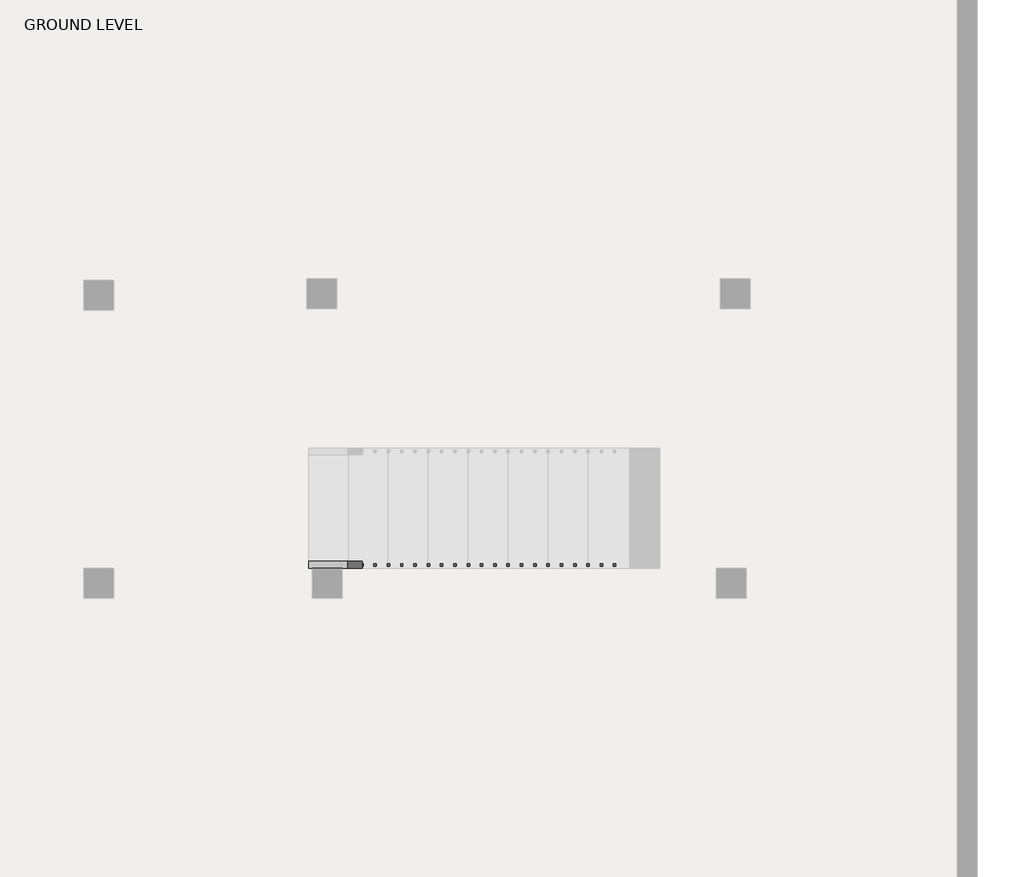
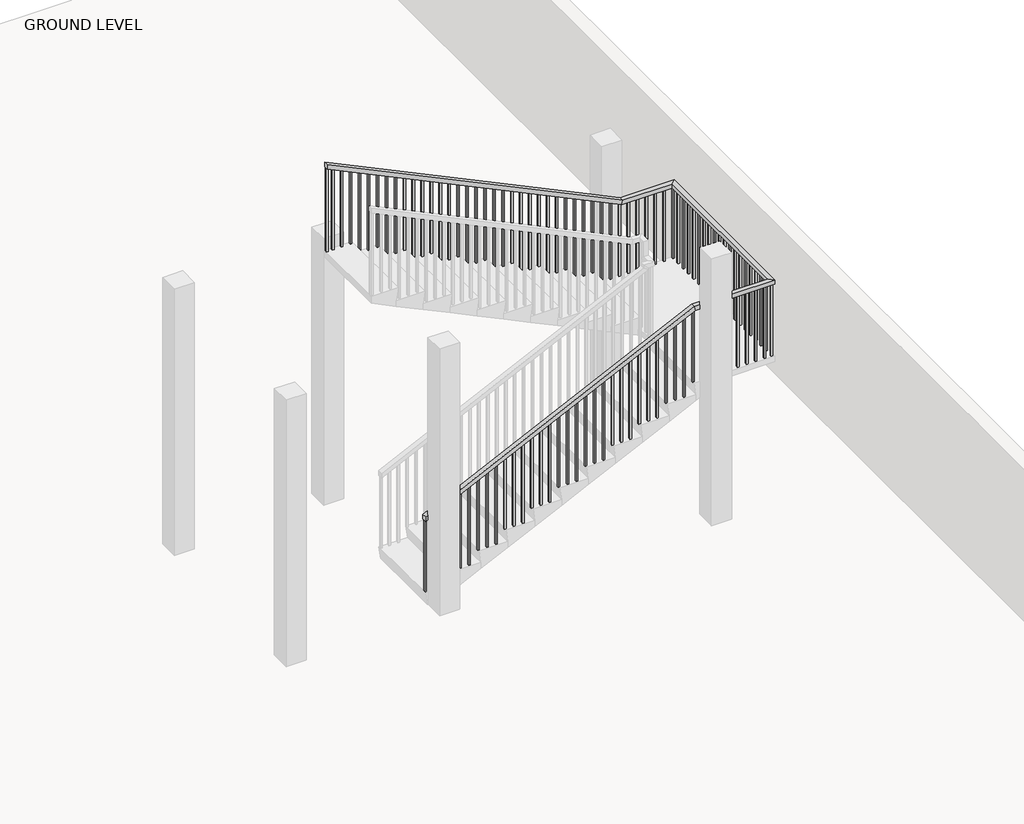
# One storey, part 2 of 3: 1 railing.
"""IFC4 building model written with IfcOpenShell, lengths in millimetres."""

from ifc_helpers import new_model, si_unit, frame, origin, place, context, project, spatial, polyline, outline, extrude, faceted_brep, element, save

model = new_model("IFC4")

# Units and contexts
model_context = context("Model", 3, world=origin())
ifc_project = project(units=[si_unit("LENGTHUNIT", "METRE", prefix="MILLI")], contexts=[model_context])

# Site, building, storey
site = spatial("IfcSite", under=ifc_project)
building = spatial("IfcBuilding", under=site)
storey = spatial("IfcBuildingStorey", under=building, Name="GROUND LEVEL", Elevation=0.0)

# Railing
placement = place(None, origin())
element("IfcRailing", 1, ObjectType="Handrail - Rectangular", at=placement, inside=storey, context=model_context, shape_type="SolidModel", body=[
    faceted_brep([(13.3134019, -453.4212413, 1059.8727273), (13.3134019, -453.4212413, 1003.5834559), (13.3134019, -504.2212413, 1003.5834559), (13.3134019, -504.2212413, 1059.8727273), (3061.3134019, -453.4212413, 2514.6), (3072.8147322, -453.4212413, 2463.8), (3072.8147322, -504.2212413, 2463.8), (3061.3134019, -504.2212413, 2514.6), (3924.9134019, -453.4212413, 2514.6), (3924.9134019, -453.4212413, 2463.8), (3975.7134019, -504.2212413, 2463.8), (3975.7134019, -504.2212413, 2514.6), (3924.9134019, 1426.1787587, 2514.6), (3924.9134019, 1426.1787587, 2463.8), (3975.7134019, 1476.9787587, 2463.8), (3975.7134019, 1476.9787587, 2514.6), (3366.1134019, 1426.1787587, 2514.6), (3354.6120715, 1426.1787587, 2463.8), (3354.6120715, 1476.9787587, 2463.8), (3366.1134019, 1476.9787587, 2514.6), (13.3134019, 1426.1787587, 4114.8), (13.3134019, 1476.9787587, 4114.8), (13.3134019, 1476.9787587, 4058.5107287), (13.3134019, 1426.1787587, 4058.5107287)], [[[0, 1, 2, 3]], [[1, 0, 4, 5]], [[2, 1, 5, 6]], [[3, 2, 6, 7]], [[0, 3, 7, 4]], [[5, 4, 8, 9]], [[6, 5, 9, 10]], [[7, 6, 10, 11]], [[4, 7, 11, 8]], [[9, 8, 12, 13]], [[10, 9, 13, 14]], [[11, 10, 14, 15]], [[8, 11, 15, 12]], [[13, 12, 16, 17]], [[14, 13, 17, 18]], [[15, 14, 18, 19]], [[12, 15, 19, 16]], [[20, 21, 22, 23]], [[17, 16, 20, 23]], [[18, 17, 23, 22]], [[19, 18, 22, 21]], [[16, 19, 21, 20]]]),
    extrude(outline(polyline([(4017.5965241, 99.0384019), (4026.6885696, 79.9884019), (3054.9272727, 79.9884019), (3054.9272727, 99.0384019), (4017.5965241, 99.0384019)])), frame((0.0, 1442.0537587, 0.0), z_axis=(0.0, 1.0, 0.0), x_axis=(0.0, 0.0, 1.0)), (0.0, 0.0, 1.0), 19.05),
    extrude(outline(polyline([(3969.105615, 200.6384019), (3978.1976605, 181.5884019), (3054.9272727, 181.5884019), (3054.9272727, 200.6384019), (3969.105615, 200.6384019)])), frame((0.0, 1442.0537587, 0.0), z_axis=(0.0, 1.0, 0.0), x_axis=(0.0, 0.0, 1.0)), (0.0, 0.0, 1.0), 19.05),
    extrude(outline(polyline([(3920.6147059, 302.2384019), (3929.7067514, 283.1884019), (3054.9272727, 283.1884019), (3054.9272727, 302.2384019), (3920.6147059, 302.2384019)])), frame((0.0, 1442.0537587, 0.0), z_axis=(0.0, 1.0, 0.0), x_axis=(0.0, 0.0, 1.0)), (0.0, 0.0, 1.0), 19.05),
    extrude(outline(polyline([(3872.1237969, 403.8384019), (3881.2158423, 384.7884019), (2909.4545455, 384.7884019), (2909.4545455, 403.8384019), (3872.1237969, 403.8384019)])), frame((0.0, 1442.0537587, 0.0), z_axis=(0.0, 1.0, 0.0), x_axis=(0.0, 0.0, 1.0)), (0.0, 0.0, 1.0), 19.05),
    extrude(outline(polyline([(3823.6328878, 505.4384019), (3832.7249332, 486.3884019), (2909.4545455, 486.3884019), (2909.4545455, 505.4384019), (3823.6328878, 505.4384019)])), frame((0.0, 1442.0537587, 0.0), z_axis=(0.0, 1.0, 0.0), x_axis=(0.0, 0.0, 1.0)), (0.0, 0.0, 1.0), 19.05),
    extrude(outline(polyline([(3775.1419787, 607.0384019), (3784.2340241, 587.9884019), (2909.4545455, 587.9884019), (2909.4545455, 607.0384019), (3775.1419787, 607.0384019)])), frame((0.0, 1442.0537587, 0.0), z_axis=(0.0, 1.0, 0.0), x_axis=(0.0, 0.0, 1.0)), (0.0, 0.0, 1.0), 19.05),
    extrude(outline(polyline([(3726.6510696, 708.6384019), (3735.743115, 689.5884019), (2763.9818182, 689.5884019), (2763.9818182, 708.6384019), (3726.6510696, 708.6384019)])), frame((0.0, 1442.0537587, 0.0), z_axis=(0.0, 1.0, 0.0), x_axis=(0.0, 0.0, 1.0)), (0.0, 0.0, 1.0), 19.05),
    extrude(outline(polyline([(3678.1601605, 810.2384019), (3687.2522059, 791.1884019), (2763.9818182, 791.1884019), (2763.9818182, 810.2384019), (3678.1601605, 810.2384019)])), frame((0.0, 1442.0537587, 0.0), z_axis=(0.0, 1.0, 0.0), x_axis=(0.0, 0.0, 1.0)), (0.0, 0.0, 1.0), 19.05),
    extrude(outline(polyline([(3629.6692514, 911.8384019), (3638.7612969, 892.7884019), (2763.9818182, 892.7884019), (2763.9818182, 911.8384019), (3629.6692514, 911.8384019)])), frame((0.0, 1442.0537587, 0.0), z_axis=(0.0, 1.0, 0.0), x_axis=(0.0, 0.0, 1.0)), (0.0, 0.0, 1.0), 19.05),
    extrude(outline(polyline([(3581.1783423, 1013.4384019), (3590.2703878, 994.3884019), (2618.5090909, 994.3884019), (2618.5090909, 1013.4384019), (3581.1783423, 1013.4384019)])), frame((0.0, 1442.0537587, 0.0), z_axis=(0.0, 1.0, 0.0), x_axis=(0.0, 0.0, 1.0)), (0.0, 0.0, 1.0), 19.05),
    extrude(outline(polyline([(3532.6874332, 1115.0384019), (3541.7794787, 1095.9884019), (2618.5090909, 1095.9884019), (2618.5090909, 1115.0384019), (3532.6874332, 1115.0384019)])), frame((0.0, 1442.0537587, 0.0), z_axis=(0.0, 1.0, 0.0), x_axis=(0.0, 0.0, 1.0)), (0.0, 0.0, 1.0), 19.05),
    extrude(outline(polyline([(3484.1965241, 1216.6384019), (3493.2885696, 1197.5884019), (2618.5090909, 1197.5884019), (2618.5090909, 1216.6384019), (3484.1965241, 1216.6384019)])), frame((0.0, 1442.0537587, 0.0), z_axis=(0.0, 1.0, 0.0), x_axis=(0.0, 0.0, 1.0)), (0.0, 0.0, 1.0), 19.05),
    extrude(outline(polyline([(3435.705615, 1318.2384019), (3444.7976605, 1299.1884019), (2473.0363636, 1299.1884019), (2473.0363636, 1318.2384019), (3435.705615, 1318.2384019)])), frame((0.0, 1442.0537587, 0.0), z_axis=(0.0, 1.0, 0.0), x_axis=(0.0, 0.0, 1.0)), (0.0, 0.0, 1.0), 19.05),
    extrude(outline(polyline([(3387.2147059, 1419.8384019), (3396.3067514, 1400.7884019), (2473.0363636, 1400.7884019), (2473.0363636, 1419.8384019), (3387.2147059, 1419.8384019)])), frame((0.0, 1442.0537587, 0.0), z_axis=(0.0, 1.0, 0.0), x_axis=(0.0, 0.0, 1.0)), (0.0, 0.0, 1.0), 19.05),
    extrude(outline(polyline([(3338.7237969, 1521.4384019), (3347.8158423, 1502.3884019), (2473.0363636, 1502.3884019), (2473.0363636, 1521.4384019), (3338.7237969, 1521.4384019)])), frame((0.0, 1442.0537587, 0.0), z_axis=(0.0, 1.0, 0.0), x_axis=(0.0, 0.0, 1.0)), (0.0, 0.0, 1.0), 19.05),
    extrude(outline(polyline([(3290.2328878, 1623.0384019), (3299.3249332, 1603.9884019), (2327.5636364, 1603.9884019), (2327.5636364, 1623.0384019), (3290.2328878, 1623.0384019)])), frame((0.0, 1442.0537587, 0.0), z_axis=(0.0, 1.0, 0.0), x_axis=(0.0, 0.0, 1.0)), (0.0, 0.0, 1.0), 19.05),
    extrude(outline(polyline([(3241.7419787, 1724.6384019), (3250.8340241, 1705.5884019), (2327.5636364, 1705.5884019), (2327.5636364, 1724.6384019), (3241.7419787, 1724.6384019)])), frame((0.0, 1442.0537587, 0.0), z_axis=(0.0, 1.0, 0.0), x_axis=(0.0, 0.0, 1.0)), (0.0, 0.0, 1.0), 19.05),
    extrude(outline(polyline([(3193.2510696, 1826.2384019), (3202.343115, 1807.1884019), (2327.5636364, 1807.1884019), (2327.5636364, 1826.2384019), (3193.2510696, 1826.2384019)])), frame((0.0, 1442.0537587, 0.0), z_axis=(0.0, 1.0, 0.0), x_axis=(0.0, 0.0, 1.0)), (0.0, 0.0, 1.0), 19.05),
    extrude(outline(polyline([(3144.7601605, 1927.8384019), (3153.8522059, 1908.7884019), (2182.0909091, 1908.7884019), (2182.0909091, 1927.8384019), (3144.7601605, 1927.8384019)])), frame((0.0, 1442.0537587, 0.0), z_axis=(0.0, 1.0, 0.0), x_axis=(0.0, 0.0, 1.0)), (0.0, 0.0, 1.0), 19.05),
    extrude(outline(polyline([(3096.2692514, 2029.4384019), (3105.3612969, 2010.3884019), (2182.0909091, 2010.3884019), (2182.0909091, 2029.4384019), (3096.2692514, 2029.4384019)])), frame((0.0, 1442.0537587, 0.0), z_axis=(0.0, 1.0, 0.0), x_axis=(0.0, 0.0, 1.0)), (0.0, 0.0, 1.0), 19.05),
    extrude(outline(polyline([(3047.7783423, 2131.0384019), (3056.8703878, 2111.9884019), (2182.0909091, 2111.9884019), (2182.0909091, 2131.0384019), (3047.7783423, 2131.0384019)])), frame((0.0, 1442.0537587, 0.0), z_axis=(0.0, 1.0, 0.0), x_axis=(0.0, 0.0, 1.0)), (0.0, 0.0, 1.0), 19.05),
    extrude(outline(polyline([(2999.2874332, 2232.6384019), (3008.3794787, 2213.5884019), (2036.6181818, 2213.5884019), (2036.6181818, 2232.6384019), (2999.2874332, 2232.6384019)])), frame((0.0, 1442.0537587, 0.0), z_axis=(0.0, 1.0, 0.0), x_axis=(0.0, 0.0, 1.0)), (0.0, 0.0, 1.0), 19.05),
    extrude(outline(polyline([(2950.7965241, 2334.2384019), (2959.8885696, 2315.1884019), (2036.6181818, 2315.1884019), (2036.6181818, 2334.2384019), (2950.7965241, 2334.2384019)])), frame((0.0, 1442.0537587, 0.0), z_axis=(0.0, 1.0, 0.0), x_axis=(0.0, 0.0, 1.0)), (0.0, 0.0, 1.0), 19.05),
    extrude(outline(polyline([(2902.305615, 2435.8384019), (2911.3976605, 2416.7884019), (2036.6181818, 2416.7884019), (2036.6181818, 2435.8384019), (2902.305615, 2435.8384019)])), frame((0.0, 1442.0537587, 0.0), z_axis=(0.0, 1.0, 0.0), x_axis=(0.0, 0.0, 1.0)), (0.0, 0.0, 1.0), 19.05),
    extrude(outline(polyline([(2853.8147059, 2537.4384019), (2862.9067514, 2518.3884019), (1891.1454545, 2518.3884019), (1891.1454545, 2537.4384019), (2853.8147059, 2537.4384019)])), frame((0.0, 1442.0537587, 0.0), z_axis=(0.0, 1.0, 0.0), x_axis=(0.0, 0.0, 1.0)), (0.0, 0.0, 1.0), 19.05),
    extrude(outline(polyline([(2805.3237969, 2639.0384019), (2814.4158423, 2619.9884019), (1891.1454545, 2619.9884019), (1891.1454545, 2639.0384019), (2805.3237969, 2639.0384019)])), frame((0.0, 1442.0537587, 0.0), z_axis=(0.0, 1.0, 0.0), x_axis=(0.0, 0.0, 1.0)), (0.0, 0.0, 1.0), 19.05),
    extrude(outline(polyline([(2756.8328878, 2740.6384019), (2765.9249332, 2721.5884019), (1891.1454545, 2721.5884019), (1891.1454545, 2740.6384019), (2756.8328878, 2740.6384019)])), frame((0.0, 1442.0537587, 0.0), z_axis=(0.0, 1.0, 0.0), x_axis=(0.0, 0.0, 1.0)), (0.0, 0.0, 1.0), 19.05),
    extrude(outline(polyline([(2708.3419787, 2842.2384019), (2717.4340241, 2823.1884019), (1745.6727273, 2823.1884019), (1745.6727273, 2842.2384019), (2708.3419787, 2842.2384019)])), frame((0.0, 1442.0537587, 0.0), z_axis=(0.0, 1.0, 0.0), x_axis=(0.0, 0.0, 1.0)), (0.0, 0.0, 1.0), 19.05),
    extrude(outline(polyline([(2659.8510696, 2943.8384019), (2668.943115, 2924.7884019), (1745.6727273, 2924.7884019), (1745.6727273, 2943.8384019), (2659.8510696, 2943.8384019)])), frame((0.0, 1442.0537587, 0.0), z_axis=(0.0, 1.0, 0.0), x_axis=(0.0, 0.0, 1.0)), (0.0, 0.0, 1.0), 19.05),
    extrude(outline(polyline([(2611.3601605, 3045.4384019), (2620.4522059, 3026.3884019), (1745.6727273, 3026.3884019), (1745.6727273, 3045.4384019), (2611.3601605, 3045.4384019)])), frame((0.0, 1442.0537587, 0.0), z_axis=(0.0, 1.0, 0.0), x_axis=(0.0, 0.0, 1.0)), (0.0, 0.0, 1.0), 19.05),
    extrude(outline(polyline([(2562.8692514, 3147.0384019), (2571.9612969, 3127.9884019), (1600.2, 3127.9884019), (1600.2, 3147.0384019), (2562.8692514, 3147.0384019)])), frame((0.0, 1442.0537587, 0.0), z_axis=(0.0, 1.0, 0.0), x_axis=(0.0, 0.0, 1.0)), (0.0, 0.0, 1.0), 19.05),
    extrude(outline(polyline([(2514.3783423, 3248.6384019), (2523.4703878, 3229.5884019), (1600.2, 3229.5884019), (1600.2, 3248.6384019), (2514.3783423, 3248.6384019)])), frame((0.0, 1442.0537587, 0.0), z_axis=(0.0, 1.0, 0.0), x_axis=(0.0, 0.0, 1.0)), (0.0, 0.0, 1.0), 19.05),
    extrude(outline(polyline([(2465.8874332, 3350.2384019), (2474.9794787, 3331.1884019), (1600.2, 3331.1884019), (1600.2, 3350.2384019), (2465.8874332, 3350.2384019)])), frame((0.0, 1442.0537587, 0.0), z_axis=(0.0, 1.0, 0.0), x_axis=(0.0, 0.0, 1.0)), (0.0, 0.0, 1.0), 19.05),
    extrude(outline(polyline([(3451.8384019, 1461.1037587), (3451.8384019, 1442.0537587), (3432.7884019, 1442.0537587), (3432.7884019, 1461.1037587), (3451.8384019, 1461.1037587)])), frame((0.0, 0.0, 1600.2), z_axis=(0.0, 0.0, 1.0), x_axis=(1.0, 0.0, 0.0)), (0.0, 0.0, 1.0), 863.6),
    extrude(outline(polyline([(3553.4384019, 1461.1037587), (3553.4384019, 1442.0537587), (3534.3884019, 1442.0537587), (3534.3884019, 1461.1037587), (3553.4384019, 1461.1037587)])), frame((0.0, 0.0, 1600.2), z_axis=(0.0, 0.0, 1.0), x_axis=(1.0, 0.0, 0.0)), (0.0, 0.0, 1.0), 863.6),
    extrude(outline(polyline([(3655.0384019, 1461.1037587), (3655.0384019, 1442.0537587), (3635.9884019, 1442.0537587), (3635.9884019, 1461.1037587), (3655.0384019, 1461.1037587)])), frame((0.0, 0.0, 1600.2), z_axis=(0.0, 0.0, 1.0), x_axis=(1.0, 0.0, 0.0)), (0.0, 0.0, 1.0), 863.6),
    extrude(outline(polyline([(3756.6384019, 1461.1037587), (3756.6384019, 1442.0537587), (3737.5884019, 1442.0537587), (3737.5884019, 1461.1037587), (3756.6384019, 1461.1037587)])), frame((0.0, 0.0, 1600.2), z_axis=(0.0, 0.0, 1.0), x_axis=(1.0, 0.0, 0.0)), (0.0, 0.0, 1.0), 863.6),
    extrude(outline(polyline([(3858.2384019, 1461.1037587), (3858.2384019, 1442.0537587), (3839.1884019, 1442.0537587), (3839.1884019, 1461.1037587), (3858.2384019, 1461.1037587)])), frame((0.0, 0.0, 1600.2), z_axis=(0.0, 0.0, 1.0), x_axis=(1.0, 0.0, 0.0)), (0.0, 0.0, 1.0), 863.6),
    extrude(outline(polyline([(3959.8384019, 1340.4537587), (3940.7884019, 1340.4537587), (3940.7884019, 1359.5037587), (3959.8384019, 1359.5037587), (3959.8384019, 1340.4537587)])), frame((0.0, 0.0, 1600.2), z_axis=(0.0, 0.0, 1.0), x_axis=(1.0, 0.0, 0.0)), (0.0, 0.0, 1.0), 863.6),
    extrude(outline(polyline([(3959.8384019, 1238.8537587), (3940.7884019, 1238.8537587), (3940.7884019, 1257.9037587), (3959.8384019, 1257.9037587), (3959.8384019, 1238.8537587)])), frame((0.0, 0.0, 1600.2), z_axis=(0.0, 0.0, 1.0), x_axis=(1.0, 0.0, 0.0)), (0.0, 0.0, 1.0), 863.6),
    extrude(outline(polyline([(3959.8384019, 1137.2537587), (3940.7884019, 1137.2537587), (3940.7884019, 1156.3037587), (3959.8384019, 1156.3037587), (3959.8384019, 1137.2537587)])), frame((0.0, 0.0, 1600.2), z_axis=(0.0, 0.0, 1.0), x_axis=(1.0, 0.0, 0.0)), (0.0, 0.0, 1.0), 863.6),
    extrude(outline(polyline([(3959.8384019, 1035.6537587), (3940.7884019, 1035.6537587), (3940.7884019, 1054.7037587), (3959.8384019, 1054.7037587), (3959.8384019, 1035.6537587)])), frame((0.0, 0.0, 1600.2), z_axis=(0.0, 0.0, 1.0), x_axis=(1.0, 0.0, 0.0)), (0.0, 0.0, 1.0), 863.6),
    extrude(outline(polyline([(3959.8384019, 934.0537587), (3940.7884019, 934.0537587), (3940.7884019, 953.1037587), (3959.8384019, 953.1037587), (3959.8384019, 934.0537587)])), frame((0.0, 0.0, 1600.2), z_axis=(0.0, 0.0, 1.0), x_axis=(1.0, 0.0, 0.0)), (0.0, 0.0, 1.0), 863.6),
    extrude(outline(polyline([(3959.8384019, 832.4537587), (3940.7884019, 832.4537587), (3940.7884019, 851.5037587), (3959.8384019, 851.5037587), (3959.8384019, 832.4537587)])), frame((0.0, 0.0, 1600.2), z_axis=(0.0, 0.0, 1.0), x_axis=(1.0, 0.0, 0.0)), (0.0, 0.0, 1.0), 863.6),
    extrude(outline(polyline([(3959.8384019, 730.8537587), (3940.7884019, 730.8537587), (3940.7884019, 749.9037587), (3959.8384019, 749.9037587), (3959.8384019, 730.8537587)])), frame((0.0, 0.0, 1600.2), z_axis=(0.0, 0.0, 1.0), x_axis=(1.0, 0.0, 0.0)), (0.0, 0.0, 1.0), 863.6),
    extrude(outline(polyline([(3959.8384019, 629.2537587), (3940.7884019, 629.2537587), (3940.7884019, 648.3037587), (3959.8384019, 648.3037587), (3959.8384019, 629.2537587)])), frame((0.0, 0.0, 1600.2), z_axis=(0.0, 0.0, 1.0), x_axis=(1.0, 0.0, 0.0)), (0.0, 0.0, 1.0), 863.6),
    extrude(outline(polyline([(3959.8384019, 527.6537587), (3940.7884019, 527.6537587), (3940.7884019, 546.7037587), (3959.8384019, 546.7037587), (3959.8384019, 527.6537587)])), frame((0.0, 0.0, 1600.2), z_axis=(0.0, 0.0, 1.0), x_axis=(1.0, 0.0, 0.0)), (0.0, 0.0, 1.0), 863.6),
    extrude(outline(polyline([(3959.8384019, 426.0537587), (3940.7884019, 426.0537587), (3940.7884019, 445.1037587), (3959.8384019, 445.1037587), (3959.8384019, 426.0537587)])), frame((0.0, 0.0, 1600.2), z_axis=(0.0, 0.0, 1.0), x_axis=(1.0, 0.0, 0.0)), (0.0, 0.0, 1.0), 863.6),
    extrude(outline(polyline([(3959.8384019, 324.4537587), (3940.7884019, 324.4537587), (3940.7884019, 343.5037587), (3959.8384019, 343.5037587), (3959.8384019, 324.4537587)])), frame((0.0, 0.0, 1600.2), z_axis=(0.0, 0.0, 1.0), x_axis=(1.0, 0.0, 0.0)), (0.0, 0.0, 1.0), 863.6),
    extrude(outline(polyline([(3959.8384019, 222.8537587), (3940.7884019, 222.8537587), (3940.7884019, 241.9037587), (3959.8384019, 241.9037587), (3959.8384019, 222.8537587)])), frame((0.0, 0.0, 1600.2), z_axis=(0.0, 0.0, 1.0), x_axis=(1.0, 0.0, 0.0)), (0.0, 0.0, 1.0), 863.6),
    extrude(outline(polyline([(3959.8384019, 121.2537587), (3940.7884019, 121.2537587), (3940.7884019, 140.3037587), (3959.8384019, 140.3037587), (3959.8384019, 121.2537587)])), frame((0.0, 0.0, 1600.2), z_axis=(0.0, 0.0, 1.0), x_axis=(1.0, 0.0, 0.0)), (0.0, 0.0, 1.0), 863.6),
    extrude(outline(polyline([(3959.8384019, 19.6537587), (3940.7884019, 19.6537587), (3940.7884019, 38.7037587), (3959.8384019, 38.7037587), (3959.8384019, 19.6537587)])), frame((0.0, 0.0, 1600.2), z_axis=(0.0, 0.0, 1.0), x_axis=(1.0, 0.0, 0.0)), (0.0, 0.0, 1.0), 863.6),
    extrude(outline(polyline([(3959.8384019, -81.9462413), (3940.7884019, -81.9462413), (3940.7884019, -62.8962413), (3959.8384019, -62.8962413), (3959.8384019, -81.9462413)])), frame((0.0, 0.0, 1600.2), z_axis=(0.0, 0.0, 1.0), x_axis=(1.0, 0.0, 0.0)), (0.0, 0.0, 1.0), 863.6),
    extrude(outline(polyline([(3959.8384019, -183.5462413), (3940.7884019, -183.5462413), (3940.7884019, -164.4962413), (3959.8384019, -164.4962413), (3959.8384019, -183.5462413)])), frame((0.0, 0.0, 1600.2), z_axis=(0.0, 0.0, 1.0), x_axis=(1.0, 0.0, 0.0)), (0.0, 0.0, 1.0), 863.6),
    extrude(outline(polyline([(3959.8384019, -285.1462413), (3940.7884019, -285.1462413), (3940.7884019, -266.0962413), (3959.8384019, -266.0962413), (3959.8384019, -285.1462413)])), frame((0.0, 0.0, 1600.2), z_axis=(0.0, 0.0, 1.0), x_axis=(1.0, 0.0, 0.0)), (0.0, 0.0, 1.0), 863.6),
    extrude(outline(polyline([(3959.8384019, -386.7462413), (3940.7884019, -386.7462413), (3940.7884019, -367.6962413), (3959.8384019, -367.6962413), (3959.8384019, -386.7462413)])), frame((0.0, 0.0, 1600.2), z_axis=(0.0, 0.0, 1.0), x_axis=(1.0, 0.0, 0.0)), (0.0, 0.0, 1.0), 863.6),
    extrude(outline(polyline([(3864.5884019, -488.3462413), (3864.5884019, -469.2962413), (3883.6384019, -469.2962413), (3883.6384019, -488.3462413), (3864.5884019, -488.3462413)])), frame((0.0, 0.0, 1600.2), z_axis=(0.0, 0.0, 1.0), x_axis=(1.0, 0.0, 0.0)), (0.0, 0.0, 1.0), 863.6),
    extrude(outline(polyline([(3762.9884019, -488.3462413), (3762.9884019, -469.2962413), (3782.0384019, -469.2962413), (3782.0384019, -488.3462413), (3762.9884019, -488.3462413)])), frame((0.0, 0.0, 1600.2), z_axis=(0.0, 0.0, 1.0), x_axis=(1.0, 0.0, 0.0)), (0.0, 0.0, 1.0), 863.6),
    extrude(outline(polyline([(3661.3884019, -488.3462413), (3661.3884019, -469.2962413), (3680.4384019, -469.2962413), (3680.4384019, -488.3462413), (3661.3884019, -488.3462413)])), frame((0.0, 0.0, 1600.2), z_axis=(0.0, 0.0, 1.0), x_axis=(1.0, 0.0, 0.0)), (0.0, 0.0, 1.0), 863.6),
    extrude(outline(polyline([(3559.7884019, -488.3462413), (3559.7884019, -469.2962413), (3578.8384019, -469.2962413), (3578.8384019, -488.3462413), (3559.7884019, -488.3462413)])), frame((0.0, 0.0, 1600.2), z_axis=(0.0, 0.0, 1.0), x_axis=(1.0, 0.0, 0.0)), (0.0, 0.0, 1.0), 863.6),
    extrude(outline(polyline([(3458.1884019, -488.3462413), (3458.1884019, -469.2962413), (3477.2384019, -469.2962413), (3477.2384019, -488.3462413), (3458.1884019, -488.3462413)])), frame((0.0, 0.0, 1600.2), z_axis=(0.0, 0.0, 1.0), x_axis=(1.0, 0.0, 0.0)), (0.0, 0.0, 1.0), 863.6),
    extrude(outline(polyline([(3356.5884019, -488.3462413), (3356.5884019, -469.2962413), (3375.6384019, -469.2962413), (3375.6384019, -488.3462413), (3356.5884019, -488.3462413)])), frame((0.0, 0.0, 1600.2), z_axis=(0.0, 0.0, 1.0), x_axis=(1.0, 0.0, 0.0)), (0.0, 0.0, 1.0), 863.6),
    extrude(outline(polyline([(3254.9884019, -488.3462413), (3254.9884019, -469.2962413), (3274.0384019, -469.2962413), (3274.0384019, -488.3462413), (3254.9884019, -488.3462413)])), frame((0.0, 0.0, 1600.2), z_axis=(0.0, 0.0, 1.0), x_axis=(1.0, 0.0, 0.0)), (0.0, 0.0, 1.0), 863.6),
    extrude(outline(polyline([(3153.3884019, -488.3462413), (3153.3884019, -469.2962413), (3172.4384019, -469.2962413), (3172.4384019, -488.3462413), (3153.3884019, -488.3462413)])), frame((0.0, 0.0, 1600.2), z_axis=(0.0, 0.0, 1.0), x_axis=(1.0, 0.0, 0.0)), (0.0, 0.0, 1.0), 863.6),
    extrude(outline(polyline([(2462.8567514, 3070.8384019), (2453.7647059, 3051.7884019), (1600.2, 3051.7884019), (1600.2, 3070.8384019), (2462.8567514, 3070.8384019)])), frame((0.0, -488.3462413, 0.0), z_axis=(0.0, 1.0, 0.0), x_axis=(0.0, 0.0, 1.0)), (0.0, 0.0, 1.0), 19.05),
    extrude(outline(polyline([(2414.3658423, 2969.2384019), (2405.2737969, 2950.1884019), (1454.7272727, 2950.1884019), (1454.7272727, 2969.2384019), (2414.3658423, 2969.2384019)])), frame((0.0, -488.3462413, 0.0), z_axis=(0.0, 1.0, 0.0), x_axis=(0.0, 0.0, 1.0)), (0.0, 0.0, 1.0), 19.05),
    extrude(outline(polyline([(2365.8749332, 2867.6384019), (2356.7828878, 2848.5884019), (1454.7272727, 2848.5884019), (1454.7272727, 2867.6384019), (2365.8749332, 2867.6384019)])), frame((0.0, -488.3462413, 0.0), z_axis=(0.0, 1.0, 0.0), x_axis=(0.0, 0.0, 1.0)), (0.0, 0.0, 1.0), 19.05),
    extrude(outline(polyline([(2317.3840241, 2766.0384019), (2308.2919787, 2746.9884019), (1454.7272727, 2746.9884019), (1454.7272727, 2766.0384019), (2317.3840241, 2766.0384019)])), frame((0.0, -488.3462413, 0.0), z_axis=(0.0, 1.0, 0.0), x_axis=(0.0, 0.0, 1.0)), (0.0, 0.0, 1.0), 19.05),
    extrude(outline(polyline([(2268.893115, 2664.4384019), (2259.8010696, 2645.3884019), (1309.2545455, 2645.3884019), (1309.2545455, 2664.4384019), (2268.893115, 2664.4384019)])), frame((0.0, -488.3462413, 0.0), z_axis=(0.0, 1.0, 0.0), x_axis=(0.0, 0.0, 1.0)), (0.0, 0.0, 1.0), 19.05),
    extrude(outline(polyline([(2220.4022059, 2562.8384019), (2211.3101605, 2543.7884019), (1309.2545455, 2543.7884019), (1309.2545455, 2562.8384019), (2220.4022059, 2562.8384019)])), frame((0.0, -488.3462413, 0.0), z_axis=(0.0, 1.0, 0.0), x_axis=(0.0, 0.0, 1.0)), (0.0, 0.0, 1.0), 19.05),
    extrude(outline(polyline([(2171.9112969, 2461.2384019), (2162.8192514, 2442.1884019), (1309.2545455, 2442.1884019), (1309.2545455, 2461.2384019), (2171.9112969, 2461.2384019)])), frame((0.0, -488.3462413, 0.0), z_axis=(0.0, 1.0, 0.0), x_axis=(0.0, 0.0, 1.0)), (0.0, 0.0, 1.0), 19.05),
    extrude(outline(polyline([(2123.4203878, 2359.6384019), (2114.3283423, 2340.5884019), (1163.7818182, 2340.5884019), (1163.7818182, 2359.6384019), (2123.4203878, 2359.6384019)])), frame((0.0, -488.3462413, 0.0), z_axis=(0.0, 1.0, 0.0), x_axis=(0.0, 0.0, 1.0)), (0.0, 0.0, 1.0), 19.05),
    extrude(outline(polyline([(2074.9294787, 2258.0384019), (2065.8374332, 2238.9884019), (1163.7818182, 2238.9884019), (1163.7818182, 2258.0384019), (2074.9294787, 2258.0384019)])), frame((0.0, -488.3462413, 0.0), z_axis=(0.0, 1.0, 0.0), x_axis=(0.0, 0.0, 1.0)), (0.0, 0.0, 1.0), 19.05),
    extrude(outline(polyline([(2026.4385696, 2156.4384019), (2017.3465241, 2137.3884019), (1163.7818182, 2137.3884019), (1163.7818182, 2156.4384019), (2026.4385696, 2156.4384019)])), frame((0.0, -488.3462413, 0.0), z_axis=(0.0, 1.0, 0.0), x_axis=(0.0, 0.0, 1.0)), (0.0, 0.0, 1.0), 19.05),
    extrude(outline(polyline([(1977.9476605, 2054.8384019), (1968.855615, 2035.7884019), (1018.3090909, 2035.7884019), (1018.3090909, 2054.8384019), (1977.9476605, 2054.8384019)])), frame((0.0, -488.3462413, 0.0), z_axis=(0.0, 1.0, 0.0), x_axis=(0.0, 0.0, 1.0)), (0.0, 0.0, 1.0), 19.05),
    extrude(outline(polyline([(1929.4567514, 1953.2384019), (1920.3647059, 1934.1884019), (1018.3090909, 1934.1884019), (1018.3090909, 1953.2384019), (1929.4567514, 1953.2384019)])), frame((0.0, -488.3462413, 0.0), z_axis=(0.0, 1.0, 0.0), x_axis=(0.0, 0.0, 1.0)), (0.0, 0.0, 1.0), 19.05),
    extrude(outline(polyline([(1880.9658423, 1851.6384019), (1871.8737969, 1832.5884019), (1018.3090909, 1832.5884019), (1018.3090909, 1851.6384019), (1880.9658423, 1851.6384019)])), frame((0.0, -488.3462413, 0.0), z_axis=(0.0, 1.0, 0.0), x_axis=(0.0, 0.0, 1.0)), (0.0, 0.0, 1.0), 19.05),
    extrude(outline(polyline([(1832.4749332, 1750.0384019), (1823.3828878, 1730.9884019), (872.8363636, 1730.9884019), (872.8363636, 1750.0384019), (1832.4749332, 1750.0384019)])), frame((0.0, -488.3462413, 0.0), z_axis=(0.0, 1.0, 0.0), x_axis=(0.0, 0.0, 1.0)), (0.0, 0.0, 1.0), 19.05),
    extrude(outline(polyline([(1783.9840241, 1648.4384019), (1774.8919787, 1629.3884019), (872.8363636, 1629.3884019), (872.8363636, 1648.4384019), (1783.9840241, 1648.4384019)])), frame((0.0, -488.3462413, 0.0), z_axis=(0.0, 1.0, 0.0), x_axis=(0.0, 0.0, 1.0)), (0.0, 0.0, 1.0), 19.05),
    extrude(outline(polyline([(1735.493115, 1546.8384019), (1726.4010696, 1527.7884019), (872.8363636, 1527.7884019), (872.8363636, 1546.8384019), (1735.493115, 1546.8384019)])), frame((0.0, -488.3462413, 0.0), z_axis=(0.0, 1.0, 0.0), x_axis=(0.0, 0.0, 1.0)), (0.0, 0.0, 1.0), 19.05),
    extrude(outline(polyline([(1687.0022059, 1445.2384019), (1677.9101605, 1426.1884019), (727.3636364, 1426.1884019), (727.3636364, 1445.2384019), (1687.0022059, 1445.2384019)])), frame((0.0, -488.3462413, 0.0), z_axis=(0.0, 1.0, 0.0), x_axis=(0.0, 0.0, 1.0)), (0.0, 0.0, 1.0), 19.05),
    extrude(outline(polyline([(1638.5112969, 1343.6384019), (1629.4192514, 1324.5884019), (727.3636364, 1324.5884019), (727.3636364, 1343.6384019), (1638.5112969, 1343.6384019)])), frame((0.0, -488.3462413, 0.0), z_axis=(0.0, 1.0, 0.0), x_axis=(0.0, 0.0, 1.0)), (0.0, 0.0, 1.0), 19.05),
    extrude(outline(polyline([(1590.0203878, 1242.0384019), (1580.9283423, 1222.9884019), (727.3636364, 1222.9884019), (727.3636364, 1242.0384019), (1590.0203878, 1242.0384019)])), frame((0.0, -488.3462413, 0.0), z_axis=(0.0, 1.0, 0.0), x_axis=(0.0, 0.0, 1.0)), (0.0, 0.0, 1.0), 19.05),
    extrude(outline(polyline([(1541.5294787, 1140.4384019), (1532.4374332, 1121.3884019), (581.8909091, 1121.3884019), (581.8909091, 1140.4384019), (1541.5294787, 1140.4384019)])), frame((0.0, -488.3462413, 0.0), z_axis=(0.0, 1.0, 0.0), x_axis=(0.0, 0.0, 1.0)), (0.0, 0.0, 1.0), 19.05),
    extrude(outline(polyline([(1493.0385696, 1038.8384019), (1483.9465241, 1019.7884019), (581.8909091, 1019.7884019), (581.8909091, 1038.8384019), (1493.0385696, 1038.8384019)])), frame((0.0, -488.3462413, 0.0), z_axis=(0.0, 1.0, 0.0), x_axis=(0.0, 0.0, 1.0)), (0.0, 0.0, 1.0), 19.05),
    extrude(outline(polyline([(1444.5476605, 937.2384019), (1435.455615, 918.1884019), (581.8909091, 918.1884019), (581.8909091, 937.2384019), (1444.5476605, 937.2384019)])), frame((0.0, -488.3462413, 0.0), z_axis=(0.0, 1.0, 0.0), x_axis=(0.0, 0.0, 1.0)), (0.0, 0.0, 1.0), 19.05),
    extrude(outline(polyline([(1396.0567514, 835.6384019), (1386.9647059, 816.5884019), (436.4181818, 816.5884019), (436.4181818, 835.6384019), (1396.0567514, 835.6384019)])), frame((0.0, -488.3462413, 0.0), z_axis=(0.0, 1.0, 0.0), x_axis=(0.0, 0.0, 1.0)), (0.0, 0.0, 1.0), 19.05),
    extrude(outline(polyline([(1347.5658423, 734.0384019), (1338.4737969, 714.9884019), (436.4181818, 714.9884019), (436.4181818, 734.0384019), (1347.5658423, 734.0384019)])), frame((0.0, -488.3462413, 0.0), z_axis=(0.0, 1.0, 0.0), x_axis=(0.0, 0.0, 1.0)), (0.0, 0.0, 1.0), 19.05),
    extrude(outline(polyline([(1299.0749332, 632.4384019), (1289.9828878, 613.3884019), (436.4181818, 613.3884019), (436.4181818, 632.4384019), (1299.0749332, 632.4384019)])), frame((0.0, -488.3462413, 0.0), z_axis=(0.0, 1.0, 0.0), x_axis=(0.0, 0.0, 1.0)), (0.0, 0.0, 1.0), 19.05),
    extrude(outline(polyline([(1250.5840241, 530.8384019), (1241.4919787, 511.7884019), (290.9454545, 511.7884019), (290.9454545, 530.8384019), (1250.5840241, 530.8384019)])), frame((0.0, -488.3462413, 0.0), z_axis=(0.0, 1.0, 0.0), x_axis=(0.0, 0.0, 1.0)), (0.0, 0.0, 1.0), 19.05),
    extrude(outline(polyline([(1202.093115, 429.2384019), (1193.0010696, 410.1884019), (290.9454545, 410.1884019), (290.9454545, 429.2384019), (1202.093115, 429.2384019)])), frame((0.0, -488.3462413, 0.0), z_axis=(0.0, 1.0, 0.0), x_axis=(0.0, 0.0, 1.0)), (0.0, 0.0, 1.0), 19.05),
    extrude(outline(polyline([(1153.6022059, 327.6384019), (1144.5101605, 308.5884019), (290.9454545, 308.5884019), (290.9454545, 327.6384019), (1153.6022059, 327.6384019)])), frame((0.0, -488.3462413, 0.0), z_axis=(0.0, 1.0, 0.0), x_axis=(0.0, 0.0, 1.0)), (0.0, 0.0, 1.0), 19.05),
    extrude(outline(polyline([(1105.1112969, 226.0384019), (1096.0192514, 206.9884019), (145.4727273, 206.9884019), (145.4727273, 226.0384019), (1105.1112969, 226.0384019)])), frame((0.0, -488.3462413, 0.0), z_axis=(0.0, 1.0, 0.0), x_axis=(0.0, 0.0, 1.0)), (0.0, 0.0, 1.0), 19.05),
    extrude(outline(polyline([(1056.6203878, 124.4384019), (1047.5283423, 105.3884019), (145.4727273, 105.3884019), (145.4727273, 124.4384019), (1056.6203878, 124.4384019)])), frame((0.0, -488.3462413, 0.0), z_axis=(0.0, 1.0, 0.0), x_axis=(0.0, 0.0, 1.0)), (0.0, 0.0, 1.0), 19.05),
    extrude(outline(polyline([(3959.8384019, 1442.0537587), (3940.7884019, 1442.0537587), (3940.7884019, 1461.1037587), (3959.8384019, 1461.1037587), (3959.8384019, 1442.0537587)])), frame((0.0, 0.0, 1600.2), z_axis=(0.0, 0.0, 1.0), x_axis=(1.0, 0.0, 0.0)), (0.0, 0.0, 1.0), 863.6),
    extrude(outline(polyline([(3940.7884019, -488.3462413), (3940.7884019, -469.2962413), (3959.8384019, -469.2962413), (3959.8384019, -488.3462413), (3940.7884019, -488.3462413)])), frame((0.0, 0.0, 1600.2), z_axis=(0.0, 0.0, 1.0), x_axis=(1.0, 0.0, 0.0)), (0.0, 0.0, 1.0), 863.6),
    extrude(outline(polyline([(4049.4186832, 32.3634019), (4058.5107287, 13.3134019), (3054.9272727, 13.3134019), (3054.9272727, 32.3634019), (4049.4186832, 32.3634019)])), frame((0.0, 1442.0537587, 0.0), z_axis=(0.0, 1.0, 0.0), x_axis=(0.0, 0.0, 1.0)), (0.0, 0.0, 1.0), 19.05),
    extrude(outline(polyline([(1012.6755014, 32.3634019), (1003.5834559, 13.3134019), (145.4727273, 13.3134019), (145.4727273, 32.3634019), (1012.6755014, 32.3634019)])), frame((0.0, -488.3462413, 0.0), z_axis=(0.0, 1.0, 0.0), x_axis=(0.0, 0.0, 1.0)), (0.0, 0.0, 1.0), 19.05),
])

save(model, "model.ifc")

# Revit data of these elements
# Type "Handrail - Rectangular"
#   Assembly Code = "C2010400"
#   built-in parameter 1008612 = 0.0416667 (stored number, unit not read)
#   built-in parameter 1008611 = 0.0416667 (stored number, unit not read)
#   built-in parameter 1008609 = 0.333333 (stored number, unit not read)
#   built-in parameter 1008604 = 0.166667 (stored number, unit not read)
#   built-in parameter 1008603 = 0.166667 (stored number, unit not read)
#   Railing Height = 3' - 0"
#   built-in parameter 1008630 = 2
#   built-in parameter 1008610 = 2
#   built-in parameter 1008618 = Baluster - Square : 3/4"
# Element 1 (IfcRailing, "Handrail - Rectangular")
#   Phase Created = New Construction
